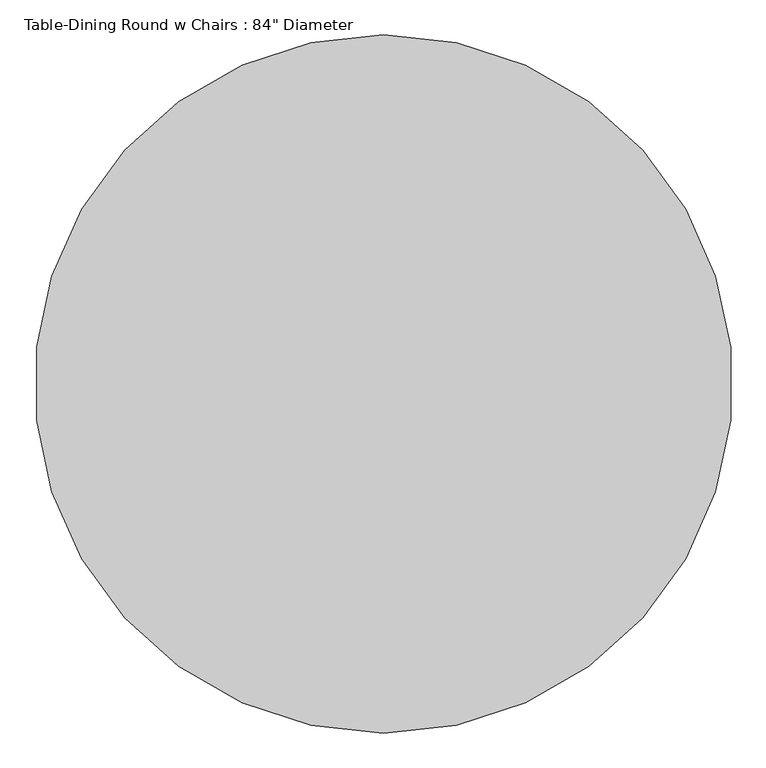
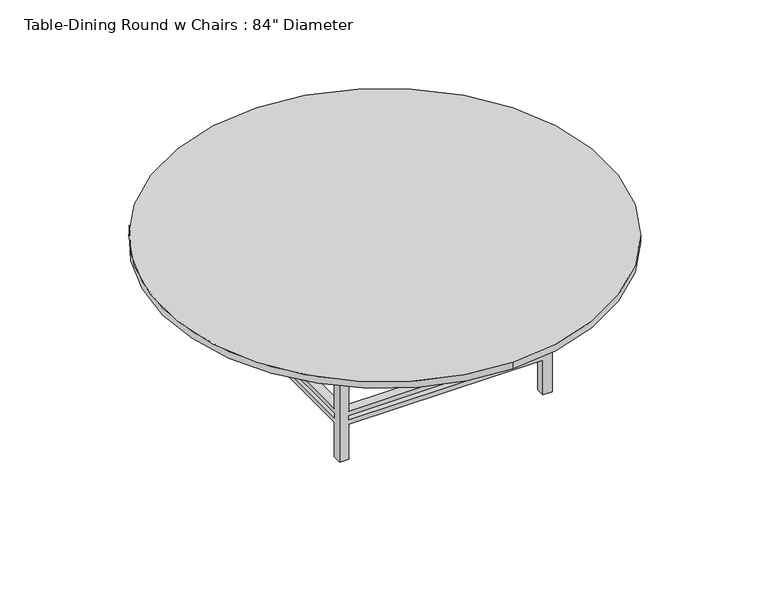
"""IFC4 building model written with IfcOpenShell, lengths in millimetres: furniture geometry."""

from ifc_helpers import new_model, si_unit, point, frame, frame_2d, origin, place, context, project, spatial, polyline, circle_curve, trimmed, segment, composite_curve, outline, extrude, faceted_brep, source, transform, mapped, element, save


def furniture_5d3b8c6f(model_context):
    return source(origin(), model_context, "Body", "SolidModel", [
        faceted_brep([(637.0819672, 348.5213115, 279.4), (637.0819672, -718.2786885, 279.4), (687.8819672, -718.2786885, 279.4), (687.8819672, 348.5213115, 279.4), (-429.7180328, -718.2786885, 279.4), (-429.7180328, -769.0786885, 279.4), (637.0819672, -769.0786885, 279.4), (-429.7180328, 348.5213115, 279.4), (-480.5180328, 348.5213115, 279.4), (-480.5180328, -718.2786885, 279.4), (637.0819672, 399.3213115, 279.4), (-429.7180328, 399.3213115, 279.4), (637.0819672, 348.5213115, 254.0), (-429.7180328, 348.5213115, 254.0), (-429.7180328, 399.3213115, 254.0), (637.0819672, 399.3213115, 254.0), (-429.7180328, -718.2786885, 254.0), (-480.5180328, -718.2786885, 254.0), (-480.5180328, 348.5213115, 254.0), (637.0819672, -718.2786885, 254.0), (637.0819672, -769.0786885, 254.0), (-429.7180328, -769.0786885, 254.0), (687.8819672, 348.5213115, 254.0), (687.8819672, -718.2786885, 254.0), (-480.5180328, 399.3213115, 647.7), (-429.7180328, 399.3213115, 647.7), (637.0819672, 399.3213115, 647.7), (687.8819672, 399.3213115, 647.7), (687.8819672, 399.3213115, 0.0), (637.0819672, 399.3213115, 0.0), (637.0819672, 399.3213115, 203.2), (-429.7180328, 399.3213115, 203.2), (-429.7180328, 399.3213115, 0.0), (-480.5180328, 399.3213115, 0.0), (-429.7180328, 399.3213115, 228.6), (637.0819672, 399.3213115, 228.6), (-480.5180328, 348.5213115, 647.7), (-480.5180328, 348.5213115, 0.0), (-480.5180328, 348.5213115, 203.2), (-480.5180328, -718.2786885, 203.2), (-480.5180328, -718.2786885, 0.0), (-480.5180328, -769.0786885, 0.0), (-480.5180328, -769.0786885, 647.7), (-480.5180328, -718.2786885, 647.7), (-480.5180328, -718.2786885, 228.6), (-480.5180328, 348.5213115, 228.6), (687.8819672, -769.0786885, 647.7), (637.0819672, -769.0786885, 647.7), (-429.7180328, -769.0786885, 647.7), (-429.7180328, -769.0786885, 0.0), (-429.7180328, -769.0786885, 203.2), (637.0819672, -769.0786885, 203.2), (637.0819672, -769.0786885, 0.0), (687.8819672, -769.0786885, 0.0), (637.0819672, -769.0786885, 228.6), (-429.7180328, -769.0786885, 228.6), (687.8819672, 348.5213115, 647.7), (687.8819672, -718.2786885, 647.7), (687.8819672, -718.2786885, 0.0), (687.8819672, -718.2786885, 203.2), (687.8819672, 348.5213115, 203.2), (687.8819672, 348.5213115, 0.0), (687.8819672, 348.5213115, 228.6), (687.8819672, -718.2786885, 228.6), (-429.7180328, 348.5213115, 647.7), (637.0819672, -718.2786885, 647.7), (637.0819672, 348.5213115, 647.7), (-429.7180328, -718.2786885, 647.7), (637.0819672, 348.5213115, 0.0), (-429.7180328, -718.2786885, 0.0), (-429.7180328, 348.5213115, 0.0), (637.0819672, -718.2786885, 0.0), (-429.7180328, 348.5213115, 228.6), (-429.7180328, 348.5213115, 203.2), (637.0819672, 348.5213115, 228.6), (637.0819672, 348.5213115, 203.2), (637.0819672, -718.2786885, 228.6), (637.0819672, -718.2786885, 203.2), (-429.7180328, -718.2786885, 228.6), (-429.7180328, -718.2786885, 203.2)], [[[0, 1, 2, 3]], [[1, 4, 5, 6]], [[4, 7, 8, 9]], [[7, 0, 10, 11]], [[12, 13, 14, 15]], [[13, 16, 17, 18]], [[16, 19, 20, 21]], [[19, 12, 22, 23]], [[24, 25, 11, 10, 26, 27, 28, 29, 30, 31, 32, 33], [14, 34, 35, 15]], [[36, 24, 33, 37, 38, 39, 40, 41, 42, 43, 9, 8], [17, 44, 45, 18]], [[46, 47, 6, 5, 48, 42, 41, 49, 50, 51, 52, 53], [20, 54, 55, 21]], [[28, 27, 56, 3, 2, 57, 46, 53, 58, 59, 60, 61], [22, 62, 63, 23]], [[1, 0, 12, 19]], [[4, 1, 19, 16]], [[7, 4, 16, 13]], [[0, 7, 13, 12]], [[25, 24, 36, 64]], [[47, 46, 57, 65]], [[26, 66, 56, 27]], [[48, 67, 43, 42]], [[29, 28, 61, 68]], [[49, 41, 40, 69]], [[32, 70, 37, 33]], [[52, 71, 58, 53]], [[13, 18, 45, 72]], [[64, 36, 8, 7]], [[37, 70, 73, 38]], [[14, 13, 72, 34]], [[25, 64, 7, 11]], [[70, 32, 31, 73]], [[12, 15, 35, 74]], [[66, 26, 10, 0]], [[29, 68, 75, 30]], [[22, 12, 74, 62]], [[56, 66, 0, 3]], [[68, 61, 60, 75]], [[19, 23, 63, 76]], [[65, 57, 2, 1]], [[58, 71, 77, 59]], [[20, 19, 76, 54]], [[47, 65, 1, 6]], [[71, 52, 51, 77]], [[16, 21, 55, 78]], [[67, 48, 5, 4]], [[49, 69, 79, 50]], [[17, 16, 78, 44]], [[43, 67, 4, 9]], [[69, 40, 39, 79]], [[74, 76, 63, 62]], [[76, 78, 55, 54]], [[78, 72, 45, 44]], [[72, 74, 35, 34]], [[75, 73, 31, 30]], [[73, 79, 39, 38]], [[79, 77, 51, 50]], [[77, 75, 60, 59]], [[76, 74, 75, 77]], [[78, 76, 77, 79]], [[72, 78, 79, 73]], [[74, 72, 73, 75]]]),
        extrude(outline(polyline([(713.2819672, 424.7213115), (713.2819672, -794.4786885), (-505.9180328, -794.4786885), (-505.9180328, 424.7213115), (713.2819672, 424.7213115)]), holes=[polyline([(687.8819672, 399.3213115), (-480.5180328, 399.3213115), (-480.5180328, -769.0786885), (687.8819672, -769.0786885), (687.8819672, 399.3213115)])]), frame((0.0, 0.0, 647.7), z_axis=(0.0, 0.0, 1.0), x_axis=(1.0, 0.0, 0.0)), (0.0, 0.0, 1.0), 76.2),
        extrude(outline(composite_curve([segment(trimmed(circle_curve(frame_2d((103.6819672, -184.8786885)), 1219.2), [point((103.6819672, -1404.0786885))], [point((103.6819672, 1034.3213115))], False, "CARTESIAN"), True, "CONTINUOUS"), segment(trimmed(circle_curve(frame_2d((103.6819672, -184.8786885)), 1219.2), [point((103.6819672, 1034.3213115))], [point((103.6819672, -1404.0786885))], False, "CARTESIAN"), True, "CONTINUOUS")], self_intersect=False)), frame((0.0, 0.0, 723.9), z_axis=(0.0, 0.0, 1.0), x_axis=(1.0, 0.0, 0.0)), (0.0, 0.0, 1.0), 38.1),
    ])


if __name__ == "__main__":
    model = new_model("IFC4")
    model_context = context("Model", 3, world=origin())
    ifc_project = project(units=[si_unit("LENGTHUNIT", "METRE", prefix="MILLI")], contexts=[model_context])
    site = spatial("IfcSite", under=ifc_project)
    building = spatial("IfcBuilding", under=site)
    placement = place(None, origin())
    furniture_shape = furniture_5d3b8c6f(model_context)
    element("IfcFurniture", 1, ObjectType="Table-Dining Round w Chairs : 84\" Diameter", at=placement, inside=building, context=model_context, shape_type="MappedRepresentation", body=[
        mapped(furniture_shape, transform((0.0, 0.0, 0.0), x_axis=(1.0, 0.0, 0.0), y_axis=(0.0, 1.0, 0.0), z_axis=(0.0, 0.0, 1.0))),
    ])
    save(model, "model.ifc")

# Revit data of these elements
# Type "Table-Dining Round w Chairs : 84\" Diameter"
#   Assembly Code = "E2020200"
#   Radius = 4' - 0"
#   Diameter = 8' - 0"
#   Height = 2' - 6"
#   Chairs = 10
#   Base Material = Pine
#   Top Material = Laminate, Linen, Matte
#   Default Elevation = 0
# Element 1 (IfcFurniture, "Table-Dining Round w Chairs : 84\" Diameter")
#   Materials on its faces: "Pine", "Laminate, Linen, Matte"
# Materials
#   "Pine": class "Wood", colour RGB 223 192 134, transparency 0, Description = "Pinus Echinata", Cost = 0
#   "Laminate, Linen, Matte": class "Plastic", colour RGB 249 239 230, transparency 0, Description = "Plastic Laminate - Linen, Matte", Cost = 0
